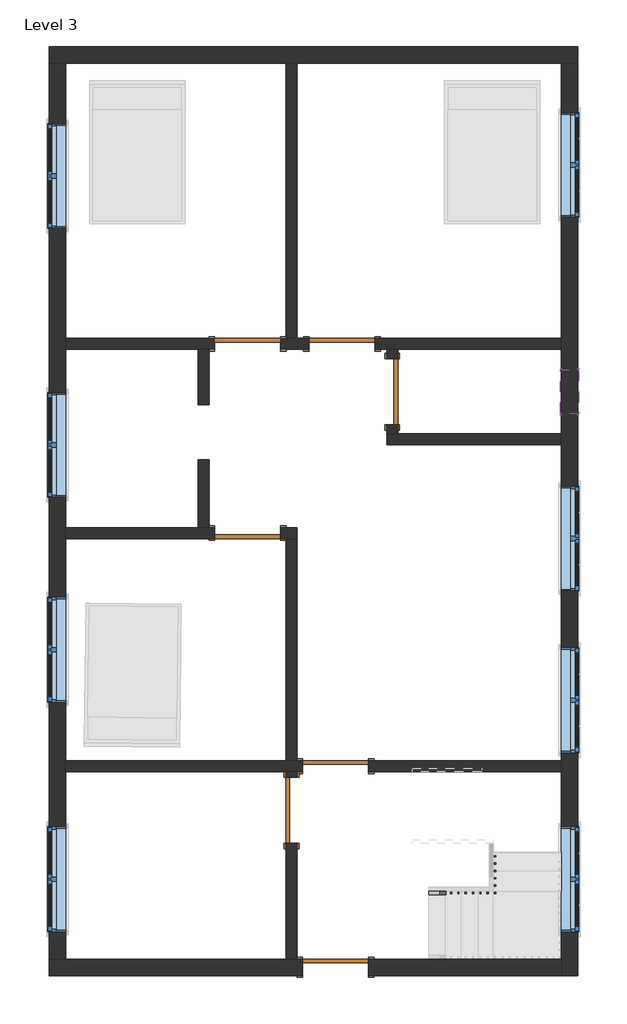
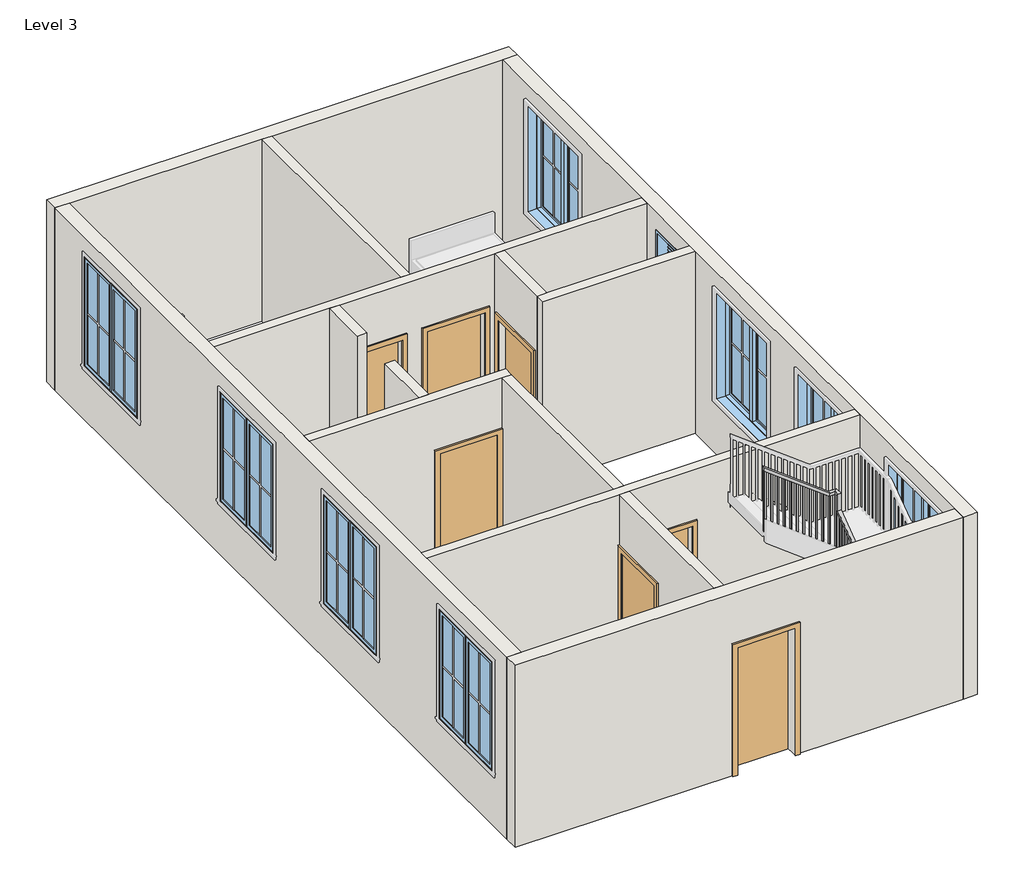
# One storey, part 1 of 2: 14 walls, 9 windows, 7 doors, 1 railing.
"""IFC4 building model written with IfcOpenShell, lengths in millimetres."""

from ifc_helpers import new_model, si_unit, frame, origin, place, context, project, spatial, polyline, outline, extrude, faceted_brep, transform, mapped, element, save
from components import door_2b0b55a0, door_686f89d2, door_16372e1c, door_a90ba1ad, window_9ac97e1a, window_f2d8fef0

model = new_model("IFC4")

# Units and contexts
model_context = context("Model", 3, world=origin())
ifc_project = project(units=[si_unit("LENGTHUNIT", "METRE", prefix="MILLI")], contexts=[model_context])

# Site, building, storey
site = spatial("IfcSite", under=ifc_project)
building = spatial("IfcBuilding", under=site)
storey = spatial("IfcBuildingStorey", under=building, Name="Level 3", Elevation=3200.4)

# Doors
placement = place(None, origin())
door_shape = door_2b0b55a0(model_context)
element("IfcDoor", 1, ObjectType="Single-Flush : 36\" x 80\"", at=placement, inside=storey, context=model_context, shape_type="MappedRepresentation", body=[
    mapped(door_shape, transform((-163.235885, 1707.4649429, 3200.4), x_axis=(0.0, 1.0, 0.0), y_axis=(-1.0, 0.0, 0.0), z_axis=(0.0, 0.0, 1.0))),
])
door_2_shape = door_686f89d2(model_context)
element("IfcDoor", 2, ObjectType="Single-Flush : 36\" x 84\"", at=placement, inside=storey, context=model_context, shape_type="MappedRepresentation", body=[
    mapped(door_2_shape, transform((-861.735885, 2367.8649429, 3200.4), x_axis=(-1.0, 0.0, 0.0), y_axis=(0.0, -1.0, 0.0), z_axis=(0.0, 0.0, 1.0))),
])
element("IfcDoor", 3, ObjectType="Single-Flush : 36\" x 84\"", at=placement, inside=storey, context=model_context, shape_type="MappedRepresentation", body=[
    mapped(door_2_shape, transform((-2169.835885, -248.3350571, 3200.4), x_axis=(1.0, 0.0, 0.0), y_axis=(0.0, 1.0, 0.0), z_axis=(0.0, 0.0, 1.0))),
])
element("IfcDoor", 4, ObjectType="Single-Flush : 36\" x 84\"", at=placement, inside=storey, context=model_context, shape_type="MappedRepresentation", body=[
    mapped(door_2_shape, transform((-950.635885, -3474.1350571, 3200.4), x_axis=(-1.0, 0.0, 0.0), y_axis=(0.0, -1.0, 0.0), z_axis=(0.0, 0.0, 1.0))),
])
door_3_shape = door_16372e1c(model_context)
element("IfcDoor", 5, ObjectType="Single-Flush : 36\" x 84\"", at=placement, inside=storey, context=model_context, shape_type="MappedRepresentation", body=[
    mapped(door_3_shape, transform((-2169.835885, 2367.8649429, 3200.4), x_axis=(1.0, 0.0, 0.0), y_axis=(0.0, 1.0, 0.0), z_axis=(0.0, 0.0, 1.0))),
])
element("IfcDoor", 6, ObjectType="Single-Flush : 36\" x 84\"", at=placement, inside=storey, context=model_context, shape_type="MappedRepresentation", body=[
    mapped(door_3_shape, transform((-1560.235885, -4083.7350571, 3200.4), x_axis=(0.0, 1.0, 0.0), y_axis=(-1.0, 0.0, 0.0), z_axis=(0.0, 0.0, 1.0))),
])
door_4_shape = door_a90ba1ad(model_context)
element("IfcDoor", 7, ObjectType="Single-Flush : 36\" x 84\"", at=placement, inside=storey, context=model_context, shape_type="MappedRepresentation", body=[
    mapped(door_4_shape, transform((-950.635885, -6255.4350571, 3200.4), x_axis=(-1.0, 0.0, 0.0), y_axis=(0.0, -1.0, 0.0), z_axis=(0.0, 0.0, 1.0))),
])

# Railing
element("IfcRailing", 8, ObjectType="Handrail - Rectangular", at=placement, inside=storey, context=model_context, shape_type="SolidModel", body=[
    faceted_brep([(344.764115, -5201.3350571, 4284.1333333), (344.764115, -5201.3350571, 4220.2686436), (344.764115, -5252.1350571, 4220.2686436), (344.764115, -5252.1350571, 4284.1333333), (1157.564115, -5201.3350571, 4903.4095238), (1208.364115, -5201.3350571, 4878.249596), (1208.364115, -5252.1350571, 4878.249596), (1157.564115, -5252.1350571, 4903.4095238), (1157.564115, -5201.3350571, 5185.2285714), (1208.364115, -5201.3350571, 5134.4285714), (1208.364115, -5252.1350571, 5134.4285714), (1157.564115, -5252.1350571, 5185.2285714), (1233.764115, -5201.3350571, 5185.2285714), (1233.764115, -5201.3350571, 5134.4285714), (1284.564115, -5252.1350571, 5134.4285714), (1284.564115, -5252.1350571, 5185.2285714), (1233.764115, -5125.1350571, 5185.2285714), (1233.764115, -5108.8554323, 5134.4285714), (1284.564115, -5108.8554323, 5134.4285714), (1284.564115, -5125.1350571, 5185.2285714), (1233.764115, -4566.3350571, 5584.3714286), (1233.764115, -4515.5350571, 5558.2288395), (1284.564115, -4515.5350571, 5558.2288395), (1284.564115, -4566.3350571, 5584.3714286), (1233.764115, -4566.3350571, 5865.8606061), (1233.764115, -4515.5350571, 5815.0606061), (1284.564115, -4515.5350571, 5815.0606061), (1284.564115, -4566.3350571, 5865.8606061), (1233.764115, -4490.1350571, 5865.8606061), (1233.764115, -4490.1350571, 5815.0606061), (1284.564115, -4439.3350571, 5815.0606061), (1284.564115, -4439.3350571, 5865.8606061), (1157.564115, -4490.1350571, 5865.8606061), (1140.4943334, -4490.1350571, 5815.0606061), (1140.4943334, -4439.3350571, 5815.0606061), (1157.564115, -4439.3350571, 5865.8606061), (116.164115, -4490.1350571, 6654.8), (116.164115, -4439.3350571, 6654.8), (116.164115, -4439.3350571, 6591.0683472), (116.164115, -4490.1350571, 6591.0683472)], [[[0, 1, 2, 3]], [[1, 0, 4, 5]], [[2, 1, 5, 6]], [[3, 2, 6, 7]], [[0, 3, 7, 4]], [[5, 4, 8, 9]], [[6, 5, 9, 10]], [[7, 6, 10, 11]], [[4, 7, 11, 8]], [[9, 8, 12, 13]], [[10, 9, 13, 14]], [[11, 10, 14, 15]], [[8, 11, 15, 12]], [[13, 12, 16, 17]], [[14, 13, 17, 18]], [[15, 14, 18, 19]], [[12, 15, 19, 16]], [[17, 16, 20, 21]], [[18, 17, 21, 22]], [[19, 18, 22, 23]], [[16, 19, 23, 20]], [[21, 20, 24, 25]], [[22, 21, 25, 26]], [[23, 22, 26, 27]], [[20, 23, 27, 24]], [[25, 24, 28, 29]], [[26, 25, 29, 30]], [[27, 26, 30, 31]], [[24, 27, 31, 28]], [[29, 28, 32, 33]], [[30, 29, 33, 34]], [[31, 30, 34, 35]], [[28, 31, 35, 32]], [[36, 37, 38, 39]], [[33, 32, 36, 39]], [[34, 33, 39, 38]], [[35, 34, 38, 37]], [[32, 35, 37, 36]]]),
    extrude(outline(polyline([(6579.0418321, 132.039115), (5571.0666667, 132.039115), (5571.0666667, 151.089115), (6564.6100139, 151.089115), (6579.0418321, 132.039115)])), frame((0.0, -4474.2600571, 0.0), z_axis=(0.0, 1.0, 0.0), x_axis=(0.0, 0.0, 1.0)), (0.0, 0.0, 1.0), 19.05),
    extrude(outline(polyline([(6502.0721351, 233.639115), (5571.0666667, 233.639115), (5571.0666667, 252.689115), (6487.6403169, 252.689115), (6502.0721351, 233.639115)])), frame((0.0, -4474.2600571, 0.0), z_axis=(0.0, 1.0, 0.0), x_axis=(0.0, 0.0, 1.0)), (0.0, 0.0, 1.0), 19.05),
    extrude(outline(polyline([(6425.1024382, 335.239115), (5571.0666667, 335.239115), (5571.0666667, 354.289115), (6410.67062, 354.289115), (6425.1024382, 335.239115)])), frame((0.0, -4474.2600571, 0.0), z_axis=(0.0, 1.0, 0.0), x_axis=(0.0, 0.0, 1.0)), (0.0, 0.0, 1.0), 19.05),
    extrude(outline(polyline([(6348.1327412, 436.839115), (5401.7333333, 436.839115), (5401.7333333, 455.889115), (6333.700923, 455.889115), (6348.1327412, 436.839115)])), frame((0.0, -4474.2600571, 0.0), z_axis=(0.0, 1.0, 0.0), x_axis=(0.0, 0.0, 1.0)), (0.0, 0.0, 1.0), 19.05),
    extrude(outline(polyline([(6271.1630442, 538.439115), (5401.7333333, 538.439115), (5401.7333333, 557.489115), (6256.731226, 557.489115), (6271.1630442, 538.439115)])), frame((0.0, -4474.2600571, 0.0), z_axis=(0.0, 1.0, 0.0), x_axis=(0.0, 0.0, 1.0)), (0.0, 0.0, 1.0), 19.05),
    extrude(outline(polyline([(6194.1933472, 640.039115), (5232.4, 640.039115), (5232.4, 659.089115), (6179.7615291, 659.089115), (6194.1933472, 640.039115)])), frame((0.0, -4474.2600571, 0.0), z_axis=(0.0, 1.0, 0.0), x_axis=(0.0, 0.0, 1.0)), (0.0, 0.0, 1.0), 19.05),
    extrude(outline(polyline([(6117.2236503, 741.639115), (5232.4, 741.639115), (5232.4, 760.689115), (6102.7918321, 760.689115), (6117.2236503, 741.639115)])), frame((0.0, -4474.2600571, 0.0), z_axis=(0.0, 1.0, 0.0), x_axis=(0.0, 0.0, 1.0)), (0.0, 0.0, 1.0), 19.05),
    extrude(outline(polyline([(6040.2539533, 843.239115), (5063.0666667, 843.239115), (5063.0666667, 862.289115), (6025.8221351, 862.289115), (6040.2539533, 843.239115)])), frame((0.0, -4474.2600571, 0.0), z_axis=(0.0, 1.0, 0.0), x_axis=(0.0, 0.0, 1.0)), (0.0, 0.0, 1.0), 19.05),
    extrude(outline(polyline([(5963.2842563, 944.839115), (5063.0666667, 944.839115), (5063.0666667, 963.889115), (5948.8524382, 963.889115), (5963.2842563, 944.839115)])), frame((0.0, -4474.2600571, 0.0), z_axis=(0.0, 1.0, 0.0), x_axis=(0.0, 0.0, 1.0)), (0.0, 0.0, 1.0), 19.05),
    extrude(outline(polyline([(5886.3145594, 1046.439115), (4893.7333333, 1046.439115), (4893.7333333, 1065.489115), (5871.8827412, 1065.489115), (5886.3145594, 1046.439115)])), frame((0.0, -4474.2600571, 0.0), z_axis=(0.0, 1.0, 0.0), x_axis=(0.0, 0.0, 1.0)), (0.0, 0.0, 1.0), 19.05),
    extrude(outline(polyline([(5809.3448624, 1148.039115), (4893.7333333, 1148.039115), (4893.7333333, 1167.089115), (5794.9130442, 1167.089115), (5809.3448624, 1148.039115)])), frame((0.0, -4474.2600571, 0.0), z_axis=(0.0, 1.0, 0.0), x_axis=(0.0, 0.0, 1.0)), (0.0, 0.0, 1.0), 19.05),
    extrude(outline(polyline([(1249.639115, -4525.0600571), (1249.639115, -4506.0100571), (1268.689115, -4506.0100571), (1268.689115, -4525.0600571), (1249.639115, -4525.0600571)])), frame((0.0, 0.0, 4555.0666667), z_axis=(0.0, 0.0, 1.0), x_axis=(1.0, 0.0, 0.0)), (0.0, 0.0, 1.0), 1259.9939394),
    extrude(outline(polyline([(-4607.6100571, 5492.4609823), (-4607.6100571, 4555.0666667), (-4626.6600571, 4555.0666667), (-4626.6600571, 5478.8538395), (-4607.6100571, 5492.4609823)])), frame((1249.639115, 0.0, 0.0), z_axis=(1.0, 0.0, 0.0), x_axis=(0.0, 1.0, 0.0)), (0.0, 0.0, 1.0), 19.05),
    extrude(outline(polyline([(-4709.2100571, 5419.8895538), (-4709.2100571, 4385.7333333), (-4728.2600571, 4385.7333333), (-4728.2600571, 5406.2824109), (-4709.2100571, 5419.8895538)])), frame((1249.639115, 0.0, 0.0), z_axis=(1.0, 0.0, 0.0), x_axis=(0.0, 1.0, 0.0)), (0.0, 0.0, 1.0), 19.05),
    extrude(outline(polyline([(-4810.8100571, 5347.3181252), (-4810.8100571, 4385.7333333), (-4829.8600571, 4385.7333333), (-4829.8600571, 5333.7109823), (-4810.8100571, 5347.3181252)])), frame((1249.639115, 0.0, 0.0), z_axis=(1.0, 0.0, 0.0), x_axis=(0.0, 1.0, 0.0)), (0.0, 0.0, 1.0), 19.05),
    extrude(outline(polyline([(-4912.4100571, 5274.7466966), (-4912.4100571, 4385.7333333), (-4931.4600571, 4385.7333333), (-4931.4600571, 5261.1395538), (-4912.4100571, 5274.7466966)])), frame((1249.639115, 0.0, 0.0), z_axis=(1.0, 0.0, 0.0), x_axis=(0.0, 1.0, 0.0)), (0.0, 0.0, 1.0), 19.05),
    extrude(outline(polyline([(-5014.0100571, 5202.1752681), (-5014.0100571, 4216.4), (-5033.0600571, 4216.4), (-5033.0600571, 5188.5681252), (-5014.0100571, 5202.1752681)])), frame((1249.639115, 0.0, 0.0), z_axis=(1.0, 0.0, 0.0), x_axis=(0.0, 1.0, 0.0)), (0.0, 0.0, 1.0), 19.05),
    extrude(outline(polyline([(-5115.6100571, 5129.6038395), (-5115.6100571, 4216.4), (-5134.6600571, 4216.4), (-5134.6600571, 5115.9966966), (-5115.6100571, 5129.6038395)])), frame((1249.639115, 0.0, 0.0), z_axis=(1.0, 0.0, 0.0), x_axis=(0.0, 1.0, 0.0)), (0.0, 0.0, 1.0), 19.05),
    extrude(outline(polyline([(4832.2876912, 1148.039115), (3877.7333333, 1148.039115), (3877.7333333, 1167.089115), (4846.8019769, 1167.089115), (4832.2876912, 1148.039115)])), frame((0.0, -5236.2600571, 0.0), z_axis=(0.0, 1.0, 0.0), x_axis=(0.0, 0.0, 1.0)), (0.0, 0.0, 1.0), 19.05),
    extrude(outline(polyline([(4754.8781674, 1046.439115), (3877.7333333, 1046.439115), (3877.7333333, 1065.489115), (4769.3924531, 1065.489115), (4754.8781674, 1046.439115)])), frame((0.0, -5236.2600571, 0.0), z_axis=(0.0, 1.0, 0.0), x_axis=(0.0, 0.0, 1.0)), (0.0, 0.0, 1.0), 19.05),
    extrude(outline(polyline([(4677.4686436, 944.839115), (3708.4, 944.839115), (3708.4, 963.889115), (4691.9829293, 963.889115), (4677.4686436, 944.839115)])), frame((0.0, -5236.2600571, 0.0), z_axis=(0.0, 1.0, 0.0), x_axis=(0.0, 0.0, 1.0)), (0.0, 0.0, 1.0), 19.05),
    extrude(outline(polyline([(4600.0591198, 843.239115), (3708.4, 843.239115), (3708.4, 862.289115), (4614.5734055, 862.289115), (4600.0591198, 843.239115)])), frame((0.0, -5236.2600571, 0.0), z_axis=(0.0, 1.0, 0.0), x_axis=(0.0, 0.0, 1.0)), (0.0, 0.0, 1.0), 19.05),
    extrude(outline(polyline([(4522.649596, 741.639115), (3539.0666667, 741.639115), (3539.0666667, 760.689115), (4537.1638817, 760.689115), (4522.649596, 741.639115)])), frame((0.0, -5236.2600571, 0.0), z_axis=(0.0, 1.0, 0.0), x_axis=(0.0, 0.0, 1.0)), (0.0, 0.0, 1.0), 19.05),
    extrude(outline(polyline([(4445.2400722, 640.039115), (3539.0666667, 640.039115), (3539.0666667, 659.089115), (4459.7543579, 659.089115), (4445.2400722, 640.039115)])), frame((0.0, -5236.2600571, 0.0), z_axis=(0.0, 1.0, 0.0), x_axis=(0.0, 0.0, 1.0)), (0.0, 0.0, 1.0), 19.05),
    extrude(outline(polyline([(4367.8305484, 538.439115), (3369.7333333, 538.439115), (3369.7333333, 557.489115), (4382.3448341, 557.489115), (4367.8305484, 538.439115)])), frame((0.0, -5236.2600571, 0.0), z_axis=(0.0, 1.0, 0.0), x_axis=(0.0, 0.0, 1.0)), (0.0, 0.0, 1.0), 19.05),
    extrude(outline(polyline([(4290.4210246, 436.839115), (3369.7333333, 436.839115), (3369.7333333, 455.889115), (4304.9353103, 455.889115), (4290.4210246, 436.839115)])), frame((0.0, -5236.2600571, 0.0), z_axis=(0.0, 1.0, 0.0), x_axis=(0.0, 0.0, 1.0)), (0.0, 0.0, 1.0), 19.05),
    extrude(outline(polyline([(1249.639115, -4474.2600571), (1249.639115, -4455.2100571), (1268.689115, -4455.2100571), (1268.689115, -4474.2600571), (1249.639115, -4474.2600571)])), frame((0.0, 0.0, 4724.4), z_axis=(0.0, 0.0, 1.0), x_axis=(1.0, 0.0, 0.0)), (0.0, 0.0, 1.0), 1090.6606061),
    extrude(outline(polyline([(1249.639115, -5217.2100571), (1268.689115, -5217.2100571), (1268.689115, -5236.2600571), (1249.639115, -5236.2600571), (1249.639115, -5217.2100571)])), frame((0.0, 0.0, 4047.0666667), z_axis=(0.0, 0.0, 1.0), x_axis=(1.0, 0.0, 0.0)), (0.0, 0.0, 1.0), 1087.3619048),
    extrude(outline(polyline([(6591.0683472, 116.164115), (5571.0666667, 116.164115), (5571.0666667, 135.214115), (6576.6365291, 135.214115), (6591.0683472, 116.164115)])), frame((0.0, -4474.2600571, 0.0), z_axis=(0.0, 1.0, 0.0), x_axis=(0.0, 0.0, 1.0)), (0.0, 0.0, 1.0), 19.05),
    extrude(outline(polyline([(4220.2686436, 344.764115), (3369.7333333, 344.764115), (3369.7333333, 363.814115), (4234.7829293, 363.814115), (4220.2686436, 344.764115)])), frame((0.0, -5236.2600571, 0.0), z_axis=(0.0, 1.0, 0.0), x_axis=(0.0, 0.0, 1.0)), (0.0, 0.0, 1.0), 19.05),
])

# Walls
element("IfcWall", 9, ObjectType="WALL 6\"", at=placement, inside=storey, context=model_context, shape_type="SweptSolid", body=[
    extrude(outline(polyline([(-1636.435885, 2444.0649429), (-1636.435885, 6254.0649429), (-1484.035885, 6254.0649429), (-1484.035885, 2444.0649429), (-1636.435885, 2444.0649429)])), frame((0.0, 0.0, 3200.4), z_axis=(0.0, 0.0, 1.0), x_axis=(1.0, 0.0, 0.0)), (0.0, 0.0, 1.0), 3048.0),
])
element("IfcWall", 10, ObjectType="WALL 6\"", at=placement, inside=storey, context=model_context, shape_type="Brep", body=[
    faceted_brep([(-1318.935885, 2444.0649429, 3200.4), (-1484.035885, 2444.0649429, 3200.4), (-1636.435885, 2444.0649429, 3200.4), (-1712.635885, 2444.0649429, 3200.4), (-1712.635885, 2444.0649429, 5334.0), (-2627.035885, 2444.0649429, 5334.0), (-2627.035885, 2444.0649429, 3200.4), (-4684.435885, 2444.0649429, 3200.4), (-4684.435885, 2444.0649429, 6248.4), (-1636.435885, 2444.0649429, 6248.4), (-1484.035885, 2444.0649429, 6248.4), (2173.564115, 2444.0649429, 6248.4), (2173.564115, 2444.0649429, 3200.4), (-404.535885, 2444.0649429, 3200.4), (-404.535885, 2444.0649429, 5334.0), (-1318.935885, 2444.0649429, 5334.0), (-1712.635885, 2291.6649429, 5334.0), (-1712.635885, 2291.6649429, 3200.4), (-1318.935885, 2291.6649429, 3200.4), (-1318.935885, 2291.6649429, 5334.0), (-404.535885, 2291.6649429, 5334.0), (-404.535885, 2291.6649429, 3200.4), (-239.435885, 2291.6649429, 3200.4), (-87.035885, 2291.6649429, 3200.4), (2173.564115, 2291.6649429, 3200.4), (2173.564115, 2291.6649429, 6248.4), (-87.035885, 2291.6649429, 6248.4), (-239.435885, 2291.6649429, 6248.4), (-2703.235885, 2291.6649429, 6248.4), (-2855.635885, 2291.6649429, 6248.4), (-4684.435885, 2291.6649429, 6248.4), (-4684.435885, 2291.6649429, 3200.4), (-2855.635885, 2291.6649429, 3200.4), (-2703.235885, 2291.6649429, 3200.4), (-2627.035885, 2291.6649429, 3200.4), (-2627.035885, 2291.6649429, 5334.0)], [[[0, 1, 2, 3, 4, 5, 6, 7, 8, 9, 10, 11, 12, 13, 14, 15]], [[16, 17, 18, 19, 20, 21, 22, 23, 24, 25, 26, 27, 28, 29, 30, 31, 32, 33, 34, 35]], [[13, 12, 24, 23, 22, 21]], [[18, 17, 3, 2, 1, 0]], [[34, 33, 32, 31, 7, 6]], [[12, 11, 25, 24]], [[8, 7, 31, 30]], [[19, 18, 0, 15]], [[20, 19, 15, 14]], [[21, 20, 14, 13]], [[4, 3, 17, 16]], [[5, 4, 16, 35]], [[6, 5, 35, 34]], [[11, 10, 9, 8, 30, 29, 28, 27, 26, 25]]]),
])
element("IfcWall", 11, ObjectType="WALL 6\"", at=placement, inside=storey, context=model_context, shape_type="SweptSolid", body=[
    extrude(outline(polyline([(-2855.635885, 1529.6649429), (-2855.635885, 2291.6649429), (-2703.235885, 2291.6649429), (-2703.235885, 1529.6649429), (-2855.635885, 1529.6649429)])), frame((0.0, 0.0, 3200.4), z_axis=(0.0, 0.0, 1.0), x_axis=(1.0, 0.0, 0.0)), (0.0, 0.0, 1.0), 3048.0),
])
element("IfcWall", 12, ObjectType="WALL 6\"", at=placement, inside=storey, context=model_context, shape_type="Brep", body=[
    faceted_brep([(-1712.635885, -324.5350571, 5334.0), (-1712.635885, -324.5350571, 3200.4), (-1636.435885, -324.5350571, 3200.4), (-1484.035885, -324.5350571, 3200.4), (-1484.035885, -324.5350571, 6248.4), (-1636.435885, -324.5350571, 6248.4), (-4684.435885, -324.5350571, 6248.4), (-4684.435885, -324.5350571, 3200.4), (-2627.035885, -324.5350571, 3200.4), (-2627.035885, -324.5350571, 5334.0), (-1484.035885, -172.1350571, 3200.4), (-1712.635885, -172.1350571, 3200.4), (-1712.635885, -172.1350571, 5334.0), (-2627.035885, -172.1350571, 5334.0), (-2627.035885, -172.1350571, 3200.4), (-2703.235885, -172.1350571, 3200.4), (-2855.635885, -172.1350571, 3200.4), (-4684.435885, -172.1350571, 3200.4), (-4684.435885, -172.1350571, 6248.4), (-2855.635885, -172.1350571, 6248.4), (-2703.235885, -172.1350571, 6248.4), (-1484.035885, -172.1350571, 6248.4)], [[[0, 1, 2, 3, 4, 5, 6, 7, 8, 9]], [[10, 11, 12, 13, 14, 15, 16, 17, 18, 19, 20, 21]], [[8, 7, 17, 16, 15, 14]], [[3, 2, 1, 11, 10]], [[7, 6, 18, 17]], [[4, 3, 10, 21]], [[12, 11, 1, 0]], [[13, 12, 0, 9]], [[14, 13, 9, 8]], [[6, 5, 4, 21, 20, 19, 18]]]),
])
element("IfcWall", 13, ObjectType="WALL 6\"", at=placement, inside=storey, context=model_context, shape_type="SweptSolid", body=[
    extrude(outline(polyline([(-1636.435885, -3397.9350571), (-1636.435885, -324.5350571), (-1484.035885, -324.5350571), (-1484.035885, -3397.9350571), (-1636.435885, -3397.9350571)])), frame((0.0, 0.0, 3200.4), z_axis=(0.0, 0.0, 1.0), x_axis=(1.0, 0.0, 0.0)), (0.0, 0.0, 1.0), 3048.0),
])
element("IfcWall", 14, ObjectType="WALL 6\"", at=placement, inside=storey, context=model_context, shape_type="Brep", body=[
    faceted_brep([(-4684.435885, -3550.3350571, 3200.4), (-1636.435885, -3550.3350571, 3200.4), (-1484.035885, -3550.3350571, 3200.4), (-1407.835885, -3550.3350571, 3200.4), (-1407.835885, -3550.3350571, 5334.0), (-493.435885, -3550.3350571, 5334.0), (-493.435885, -3550.3350571, 3200.4), (2173.564115, -3550.3350571, 3200.4), (2173.564115, -3550.3350571, 6248.4), (-1484.035885, -3550.3350571, 6248.4), (-1636.435885, -3550.3350571, 6248.4), (-4684.435885, -3550.3350571, 6248.4), (-1407.835885, -3397.9350571, 5334.0), (-1407.835885, -3397.9350571, 3200.4), (-1484.035885, -3397.9350571, 3200.4), (-1636.435885, -3397.9350571, 3200.4), (-4684.435885, -3397.9350571, 3200.4), (-4684.435885, -3397.9350571, 6248.4), (-1636.435885, -3397.9350571, 6248.4), (-1484.035885, -3397.9350571, 6248.4), (2173.564115, -3397.9350571, 6248.4), (2173.564115, -3397.9350571, 3200.4), (-493.435885, -3397.9350571, 3200.4), (-493.435885, -3397.9350571, 5334.0)], [[[0, 1, 2, 3, 4, 5, 6, 7, 8, 9, 10, 11]], [[12, 13, 14, 15, 16, 17, 18, 19, 20, 21, 22, 23]], [[22, 21, 7, 6]], [[16, 15, 14, 13, 3, 2, 1, 0]], [[8, 7, 21, 20]], [[0, 11, 17, 16]], [[4, 3, 13, 12]], [[5, 4, 12, 23]], [[6, 5, 23, 22]], [[11, 10, 9, 8, 20, 19, 18, 17]]]),
])
element("IfcWall", 15, ObjectType="WALL 6\"", at=placement, inside=storey, context=model_context, shape_type="SweptSolid", body=[
    extrude(outline(polyline([(-3550.3350571, 3200.4), (-3626.5350571, 3200.4), (-3626.5350571, 5334.0), (-4540.9350571, 5334.0), (-4540.9350571, 3200.4), (-6141.1350571, 3200.4), (-6141.1350571, 6248.4), (-3550.3350571, 6248.4), (-3550.3350571, 3200.4)])), frame((-1636.435885, 0.0, 0.0), z_axis=(1.0, 0.0, 0.0), x_axis=(0.0, 1.0, 0.0)), (0.0, 0.0, 1.0), 152.4),
])
element("IfcWall", 16, ObjectType="WALL 6\"", at=placement, inside=storey, context=model_context, shape_type="Brep", body=[
    faceted_brep([(2173.564115, 1123.2649429, 3200.4), (-87.035885, 1123.2649429, 3200.4), (-239.435885, 1123.2649429, 3200.4), (-239.435885, 1123.2649429, 6248.4), (-87.035885, 1123.2649429, 6248.4), (2173.564115, 1123.2649429, 6248.4), (2173.564115, 970.8649429, 3200.4), (2173.564115, 970.8649429, 6248.4), (-239.435885, 970.8649429, 6248.4), (-239.435885, 970.8649429, 3200.4)], [[[0, 1, 2, 3, 4, 5]], [[6, 7, 8, 9]], [[2, 1, 0, 6, 9]], [[0, 5, 7, 6]], [[3, 2, 9, 8]], [[5, 4, 3, 8, 7]]]),
])
element("IfcWall", 17, ObjectType="WALL 6\"", at=placement, inside=storey, context=model_context, shape_type="SweptSolid", body=[
    extrude(outline(polyline([(2291.6649429, 3200.4), (2164.6649429, 3200.4), (2164.6649429, 5232.4), (1250.2649429, 5232.4), (1250.2649429, 3200.4), (1123.2649429, 3200.4), (1123.2649429, 6248.4), (2291.6649429, 6248.4), (2291.6649429, 3200.4)])), frame((-239.435885, 0.0, 0.0), z_axis=(1.0, 0.0, 0.0), x_axis=(0.0, 1.0, 0.0)), (0.0, 0.0, 1.0), 152.4),
])
element("IfcWall", 18, ObjectType="WALL 6\"", at=placement, inside=storey, context=model_context, shape_type="SweptSolid", body=[
    extrude(outline(polyline([(-2855.635885, -172.1350571), (-2855.635885, 767.6649429), (-2703.235885, 767.6649429), (-2703.235885, -172.1350571), (-2855.635885, -172.1350571)])), frame((0.0, 0.0, 3200.4), z_axis=(0.0, 0.0, 1.0), x_axis=(1.0, 0.0, 0.0)), (0.0, 0.0, 1.0), 3048.0),
])
element("IfcWall", 19, ObjectType="WALL 9\"", at=placement, inside=storey, context=model_context, shape_type="Brep", body=[
    faceted_brep([(-4913.035885, 6254.0649429, 3200.4), (-4684.435885, 6254.0649429, 3200.4), (-1636.435885, 6254.0649429, 3200.4), (-1484.035885, 6254.0649429, 3200.4), (2173.564115, 6254.0649429, 3200.4), (2402.164115, 6254.0649429, 3200.4), (2402.164115, 6254.0649429, 6248.4), (2173.564115, 6254.0649429, 6248.4), (-1484.035885, 6254.0649429, 6248.4), (-1636.435885, 6254.0649429, 6248.4), (-4684.435885, 6254.0649429, 6248.4), (-4913.035885, 6254.0649429, 6248.4), (-4913.035885, 6482.6649429, 3200.4), (-4913.035885, 6482.6649429, 6248.4), (2402.164115, 6482.6649429, 6248.4), (2402.164115, 6482.6649429, 3200.4)], [[[0, 1, 2, 3, 4, 5, 6, 7, 8, 9, 10, 11]], [[12, 13, 14, 15]], [[5, 4, 3, 2, 1, 0, 12, 15]], [[6, 5, 15, 14]], [[0, 11, 13, 12]], [[11, 10, 9, 8, 7, 6, 14, 13]]]),
])
element("IfcWall", 20, ObjectType="WALL 9\"", at=placement, inside=storey, context=model_context, shape_type="Brep", body=[
    faceted_brep([(2173.564115, 6254.0649429, 3200.4), (2173.564115, 2444.0649429, 3200.4), (2173.564115, 2291.6649429, 3200.4), (2173.564115, 1123.2649429, 3200.4), (2173.564115, 970.8649429, 3200.4), (2173.564115, -3397.9350571, 3200.4), (2173.564115, -3550.3350571, 3200.4), (2173.564115, -6141.1350571, 3200.4), (2173.564115, -6369.7350571, 3200.4), (2173.564115, -6369.7350571, 6248.4), (2173.564115, -6141.1350571, 6248.4), (2173.564115, -3550.3350571, 6248.4), (2173.564115, -3397.9350571, 6248.4), (2173.564115, 970.8649429, 6248.4), (2173.564115, 1123.2649429, 6248.4), (2173.564115, 2291.6649429, 6248.4), (2173.564115, 2444.0649429, 6248.4), (2173.564115, 6254.0649429, 6248.4), (2173.564115, -5760.1350571, 5943.6), (2173.564115, -5760.1350571, 4114.8), (2173.564115, -4312.3350571, 4114.8), (2173.564115, -4312.3350571, 5943.6), (2173.564115, -3283.6350571, 5943.6), (2173.564115, -3283.6350571, 4114.8), (2173.564115, -1835.8350571, 4114.8), (2173.564115, -1835.8350571, 5943.6), (2173.564115, -1048.4350571, 5943.6), (2173.564115, -1048.4350571, 4114.8), (2173.564115, 399.3649429, 4114.8), (2173.564115, 399.3649429, 5943.6), (2173.564115, 4120.4649429, 5943.6), (2173.564115, 4120.4649429, 4114.8), (2173.564115, 5568.2649429, 4114.8), (2173.564115, 5568.2649429, 5943.6), (2173.564115, 2012.2649429, 5943.6), (2173.564115, 1402.6649429, 5943.6), (2173.564115, 1402.6649429, 5334.0), (2173.564115, 2012.2649429, 5334.0), (2402.164115, 6254.0649429, 3200.4), (2402.164115, 6254.0649429, 6248.4), (2402.164115, -6369.7350571, 6248.4), (2402.164115, -6369.7350571, 3200.4), (2402.164115, -5760.1350571, 5943.6), (2402.164115, -4312.3350571, 5943.6), (2402.164115, -4312.3350571, 4114.8), (2402.164115, -5760.1350571, 4114.8), (2402.164115, -3283.6350571, 5943.6), (2402.164115, -1835.8350571, 5943.6), (2402.164115, -1835.8350571, 4114.8), (2402.164115, -3283.6350571, 4114.8), (2402.164115, -1048.4350571, 5943.6), (2402.164115, 399.3649429, 5943.6), (2402.164115, 399.3649429, 4114.8), (2402.164115, -1048.4350571, 4114.8), (2402.164115, 4120.4649429, 5943.6), (2402.164115, 5568.2649429, 5943.6), (2402.164115, 5568.2649429, 4114.8), (2402.164115, 4120.4649429, 4114.8), (2402.164115, 2012.2649429, 5943.6), (2402.164115, 2012.2649429, 5334.0), (2402.164115, 1402.6649429, 5334.0), (2402.164115, 1402.6649429, 5943.6)], [[[0, 1, 2, 3, 4, 5, 6, 7, 8, 9, 10, 11, 12, 13, 14, 15, 16, 17], [18, 19, 20, 21], [22, 23, 24, 25], [26, 27, 28, 29], [30, 31, 32, 33], [34, 35, 36, 37]], [[38, 39, 40, 41], [42, 43, 44, 45], [46, 47, 48, 49], [50, 51, 52, 53], [54, 55, 56, 57], [58, 59, 60, 61]], [[8, 7, 6, 5, 4, 3, 2, 1, 0, 38, 41]], [[0, 17, 39, 38]], [[9, 8, 41, 40]], [[19, 18, 42, 45]], [[20, 19, 45, 44]], [[21, 20, 44, 43]], [[18, 21, 43, 42]], [[23, 22, 46, 49]], [[24, 23, 49, 48]], [[25, 24, 48, 47]], [[22, 25, 47, 46]], [[27, 26, 50, 53]], [[28, 27, 53, 52]], [[29, 28, 52, 51]], [[26, 29, 51, 50]], [[31, 30, 54, 57]], [[32, 31, 57, 56]], [[33, 32, 56, 55]], [[30, 33, 55, 54]], [[59, 58, 34, 37]], [[60, 59, 37, 36]], [[61, 60, 36, 35]], [[58, 61, 35, 34]], [[17, 16, 15, 14, 13, 12, 11, 10, 9, 40, 39]]]),
])
element("IfcWall", 21, ObjectType="WALL 9\"", at=placement, inside=storey, context=model_context, shape_type="Brep", body=[
    faceted_brep([(-1407.835885, -6141.1350571, 5334.0), (-1407.835885, -6141.1350571, 3200.4), (-1484.035885, -6141.1350571, 3200.4), (-1636.435885, -6141.1350571, 3200.4), (-4684.435885, -6141.1350571, 3200.4), (-4913.035885, -6141.1350571, 3200.4), (-4913.035885, -6141.1350571, 6248.4), (-4684.435885, -6141.1350571, 6248.4), (-1636.435885, -6141.1350571, 6248.4), (-1484.035885, -6141.1350571, 6248.4), (2173.564115, -6141.1350571, 6248.4), (2173.564115, -6141.1350571, 3200.4), (-493.435885, -6141.1350571, 3200.4), (-493.435885, -6141.1350571, 5334.0), (-4913.035885, -6369.7350571, 3200.4), (-1407.835885, -6369.7350571, 3200.4), (-1407.835885, -6369.7350571, 5334.0), (-493.435885, -6369.7350571, 5334.0), (-493.435885, -6369.7350571, 3200.4), (2173.564115, -6369.7350571, 3200.4), (2173.564115, -6369.7350571, 6248.4), (-4913.035885, -6369.7350571, 6248.4)], [[[0, 1, 2, 3, 4, 5, 6, 7, 8, 9, 10, 11, 12, 13]], [[14, 15, 16, 17, 18, 19, 20, 21]], [[12, 11, 19, 18]], [[5, 4, 3, 2, 1, 15, 14]], [[11, 10, 20, 19]], [[6, 5, 14, 21]], [[16, 15, 1, 0]], [[17, 16, 0, 13]], [[18, 17, 13, 12]], [[10, 9, 8, 7, 6, 21, 20]]]),
])
element("IfcWall", 22, ObjectType="WALL 9\"", at=placement, inside=storey, context=model_context, shape_type="Brep", body=[
    faceted_brep([(-4684.435885, -6141.1350571, 3200.4), (-4684.435885, -3550.3350571, 3200.4), (-4684.435885, -3397.9350571, 3200.4), (-4684.435885, -324.5350571, 3200.4), (-4684.435885, -172.1350571, 3200.4), (-4684.435885, 2291.6649429, 3200.4), (-4684.435885, 2444.0649429, 3200.4), (-4684.435885, 6254.0649429, 3200.4), (-4684.435885, 6254.0649429, 6248.4), (-4684.435885, 2444.0649429, 6248.4), (-4684.435885, 2291.6649429, 6248.4), (-4684.435885, -172.1350571, 6248.4), (-4684.435885, -324.5350571, 6248.4), (-4684.435885, -3397.9350571, 6248.4), (-4684.435885, -3550.3350571, 6248.4), (-4684.435885, -6141.1350571, 6248.4), (-4684.435885, -4312.3350571, 5943.6), (-4684.435885, -4312.3350571, 4114.8), (-4684.435885, -5760.1350571, 4114.8), (-4684.435885, -5760.1350571, 5943.6), (-4684.435885, -1137.3350571, 5943.6), (-4684.435885, -1137.3350571, 4114.8), (-4684.435885, -2585.1350571, 4114.8), (-4684.435885, -2585.1350571, 5943.6), (-4684.435885, 1694.7649429, 5943.6), (-4684.435885, 1694.7649429, 4114.8), (-4684.435885, 246.9649429, 4114.8), (-4684.435885, 246.9649429, 5943.6), (-4684.435885, 5415.8649429, 5943.6), (-4684.435885, 5415.8649429, 4114.8), (-4684.435885, 3968.0649429, 4114.8), (-4684.435885, 3968.0649429, 5943.6), (-4913.035885, -6141.1350571, 3200.4), (-4913.035885, -6141.1350571, 6248.4), (-4913.035885, 6254.0649429, 6248.4), (-4913.035885, 6254.0649429, 3200.4), (-4913.035885, -4312.3350571, 5943.6), (-4913.035885, -5760.1350571, 5943.6), (-4913.035885, -5760.1350571, 4114.8), (-4913.035885, -4312.3350571, 4114.8), (-4913.035885, -1137.3350571, 5943.6), (-4913.035885, -2585.1350571, 5943.6), (-4913.035885, -2585.1350571, 4114.8), (-4913.035885, -1137.3350571, 4114.8), (-4913.035885, 1694.7649429, 5943.6), (-4913.035885, 246.9649429, 5943.6), (-4913.035885, 246.9649429, 4114.8), (-4913.035885, 1694.7649429, 4114.8), (-4913.035885, 5415.8649429, 5943.6), (-4913.035885, 3968.0649429, 5943.6), (-4913.035885, 3968.0649429, 4114.8), (-4913.035885, 5415.8649429, 4114.8)], [[[0, 1, 2, 3, 4, 5, 6, 7, 8, 9, 10, 11, 12, 13, 14, 15], [16, 17, 18, 19], [20, 21, 22, 23], [24, 25, 26, 27], [28, 29, 30, 31]], [[32, 33, 34, 35], [36, 37, 38, 39], [40, 41, 42, 43], [44, 45, 46, 47], [48, 49, 50, 51]], [[7, 6, 5, 4, 3, 2, 1, 0, 32, 35]], [[8, 7, 35, 34]], [[0, 15, 33, 32]], [[17, 16, 36, 39]], [[18, 17, 39, 38]], [[19, 18, 38, 37]], [[16, 19, 37, 36]], [[21, 20, 40, 43]], [[22, 21, 43, 42]], [[23, 22, 42, 41]], [[20, 23, 41, 40]], [[25, 24, 44, 47]], [[26, 25, 47, 46]], [[27, 26, 46, 45]], [[24, 27, 45, 44]], [[29, 28, 48, 51]], [[30, 29, 51, 50]], [[31, 30, 50, 49]], [[28, 31, 49, 48]], [[15, 14, 13, 12, 11, 10, 9, 8, 34, 33]]]),
])

# Windows
window_shape = window_9ac97e1a(model_context)
element("IfcWindow", 23, ObjectType="Window-Casement-Double : 57\" x 72\"", at=placement, inside=storey, context=model_context, shape_type="MappedRepresentation", body=[
    mapped(window_shape, transform((-4798.735885, -5036.2350571, 3200.4), x_axis=(0.0, 1.0, 0.0), y_axis=(-1.0, 0.0, 0.0), z_axis=(0.0, 0.0, 1.0))),
])
element("IfcWindow", 24, ObjectType="Window-Casement-Double : 57\" x 72\"", at=placement, inside=storey, context=model_context, shape_type="MappedRepresentation", body=[
    mapped(window_shape, transform((2287.864115, -5036.2350571, 3200.4), x_axis=(0.0, -1.0, 0.0), y_axis=(1.0, 0.0, 0.0), z_axis=(0.0, 0.0, 1.0))),
])
element("IfcWindow", 25, ObjectType="Window-Casement-Double : 57\" x 72\"", at=placement, inside=storey, context=model_context, shape_type="MappedRepresentation", body=[
    mapped(window_shape, transform((2287.864115, -2559.7350571, 3200.4), x_axis=(0.0, -1.0, 0.0), y_axis=(1.0, 0.0, 0.0), z_axis=(0.0, 0.0, 1.0))),
])
element("IfcWindow", 26, ObjectType="Window-Casement-Double : 57\" x 72\"", at=placement, inside=storey, context=model_context, shape_type="MappedRepresentation", body=[
    mapped(window_shape, transform((2287.864115, -324.5350571, 3200.4), x_axis=(0.0, -1.0, 0.0), y_axis=(1.0, 0.0, 0.0), z_axis=(0.0, 0.0, 1.0))),
])
element("IfcWindow", 27, ObjectType="Window-Casement-Double : 57\" x 72\"", at=placement, inside=storey, context=model_context, shape_type="MappedRepresentation", body=[
    mapped(window_shape, transform((-4798.735885, -1861.2350571, 3200.4), x_axis=(0.0, 1.0, 0.0), y_axis=(-1.0, 0.0, 0.0), z_axis=(0.0, 0.0, 1.0))),
])
element("IfcWindow", 28, ObjectType="Window-Casement-Double : 57\" x 72\"", at=placement, inside=storey, context=model_context, shape_type="MappedRepresentation", body=[
    mapped(window_shape, transform((-4798.735885, 970.8649429, 3200.4), x_axis=(0.0, 1.0, 0.0), y_axis=(-1.0, 0.0, 0.0), z_axis=(0.0, 0.0, 1.0))),
])
element("IfcWindow", 29, ObjectType="Window-Casement-Double : 57\" x 72\"", at=placement, inside=storey, context=model_context, shape_type="MappedRepresentation", body=[
    mapped(window_shape, transform((-4798.735885, 4691.9649429, 3200.4), x_axis=(0.0, 1.0, 0.0), y_axis=(-1.0, 0.0, 0.0), z_axis=(0.0, 0.0, 1.0))),
])
element("IfcWindow", 30, ObjectType="Window-Casement-Double : 57\" x 72\"", at=placement, inside=storey, context=model_context, shape_type="MappedRepresentation", body=[
    mapped(window_shape, transform((2287.864115, 4844.3649429, 3200.4), x_axis=(0.0, -1.0, 0.0), y_axis=(1.0, 0.0, 0.0), z_axis=(0.0, 0.0, 1.0))),
])
window_2_shape = window_f2d8fef0(model_context)
element("IfcWindow", 31, ObjectType="Window-Louvers : 24\" x 24\"", at=placement, inside=storey, context=model_context, shape_type="MappedRepresentation", body=[
    mapped(window_2_shape, transform((2294.214115, 1707.4649429, 4419.6), x_axis=(0.0, -1.0, 0.0), y_axis=(1.0, 0.0, 0.0), z_axis=(0.0, 0.0, 1.0))),
])

save(model, "model.ifc")

# Revit data of these elements
# Type "Single-Flush : 36\" x 80\""
#   Type Mark = "6"
#   Construction Type Id = "MDOOR"
#   Assembly Code = "C1020"
#   Analytic Construction = "Metal"
#   Thickness = 0' - 2"
#   Heat Transfer Coefficient (U) = 0.651978 BTU/(h·ft²·°F)
#   Height = 6' - 8"
#   Trim Projection Ext = 0' - 1"
#   Trim Projection Int = 0' - 1"
#   Trim Width = 0' - 3"
#   Width = 3' - 0"
#   Define Thermal Properties by = 1
#   Define Thermal Properties by = 1
#   Door Material = Door - Panel
#   Frame Material = Door - Frame
#   Visual Light Transmittance = 0
#   Solar Heat Gain Coefficient = 0
#   Function = (empty or 0)
#   Wall Closure = (empty or 0)
# Type "Single-Flush : 36\" x 84\""
#   Type Mark = "1"
#   Construction Type Id = "MDOOR"
#   Assembly Code = "C1020"
#   Analytic Construction = "Metal"
#   Thickness = 0' - 2"
#   Heat Transfer Coefficient (U) = 0.651978 BTU/(h·ft²·°F)
#   Height = 7' - 0"
#   Trim Projection Ext = 0' - 1"
#   Trim Projection Int = 0' - 1"
#   Trim Width = 0' - 3"
#   Width = 3' - 0"
#   Define Thermal Properties by = 1
#   Define Thermal Properties by = 1
#   Door Material = Door - Panel
#   Frame Material = Door - Frame
#   Visual Light Transmittance = 0
#   Solar Heat Gain Coefficient = 0
#   Function = (empty or 0)
#   Wall Closure = (empty or 0)
# Type "Handrail - Rectangular"
#   Assembly Code = "C2010400"
#   built-in parameter 1008612 = 0.0416667 (stored number, unit not read)
#   built-in parameter 1008611 = 0.0416667 (stored number, unit not read)
#   built-in parameter 1008609 = 0.333333 (stored number, unit not read)
#   built-in parameter 1008604 = 0.166667 (stored number, unit not read)
#   built-in parameter 1008603 = 0.166667 (stored number, unit not read)
#   Railing Height = 3' - 0"
#   built-in parameter 1008630 = 2
#   built-in parameter 1008610 = 2
#   built-in parameter 1008618 = Baluster - Square : 3/4"
# Type "WALL 6\""
#   Assembly Code = "B2010"
#   Layers, outside or top first: 0' - 6" no material (function 1)
# Type "WALL 9\""
#   Assembly Code = "B2010"
#   Layers, outside or top first: 0' - 9" no material (function 1)
# Type "Window-Casement-Double : 57\" x 72\""
#   Type Mark = "17"
#   Fire Rating = "0.5h"
#   Assembly Code = "B2020100"
#   Analytic Construction = "Double glazing - domestic"
#   Frame Extension [instance default] = 0' - 0 1/4"
#   Window Inset [instance default] = 0' - 0"
#   Wall Thickness [instance default] = 0' - 6"
#   Interior Wall Closure [instance default] = 0' - 2 1/4"
#   Half Width = 2' - 4 1/2"
#   Visual Light Transmittance = 0.81
#   Thermal Resistance (R) = 1.8146 (h·ft²·°F)/BTU
#   Solar Heat Gain Coefficient = 0.76
#   Rough Width = 4' - 9 1/2"
#   Rough Height = 6' - 0 1/2"
#   Height = 6' - 0"
#   Heat Transfer Coefficient (U) = 0.5511 BTU/(h·ft²·°F)
#   Exterior Wall Closure [instance default] = 0' - 1 1/4"
#   Extension Jamb [instance default] = 0' - 2 1/4"
#   Default Sill Height = 3' - 0"
#   Width = 4' - 9"
#   Define Thermal Properties by = 0
#   Muntin Visibility = yes
#   Interior Trim Visibility [instance default] = yes
#   Exterior Trim Visibility [instance default] = yes
#   Extension Jamb Visibility [instance default] = yes
#   Interior Trim Material = Wood - Stained
#   Muntin Pattern = Muntin Pattern_2x2 : Muntin Pattern_2x2
#   Interior Trim = Trim-Window-Interior-Flat : Picture Frame
#   Interior Frame Material = Wood - Stained
#   Glass Panel Material = Glass
#   Exterior Trim Material = Clad - White
#   Exterior Trim = Trim-Window-Exterior-Flat : with Sill
#   Exterior Frame Material = Clad - White
#   Wall Closure = (empty or 0)
# Type "Window-Louvers : 24\" x 24\""
#   Type Mark = "18"
#   Construction Type Id = "GSP4R"
#   Assembly Code = "B20"
#   Analytic Construction = "1/8 in Pilkington single glazing"
#   Visual Light Transmittance = 0.9
#   Thermal Resistance (R) = 1.53941 (h·ft²·°F)/BTU
#   Solar Heat Gain Coefficient = 0.78
#   Max Height = 1' - 11.74264"
#   Height = 2' - 0"
#   Heat Transfer Coefficient (U) = 0.6496 BTU/(h·ft²·°F)
#   Blade Width [instance default] = 1' - 10 1/2"
#   Blade Vertical Thickness = 0' - 0.35355"
#   Blade Thickness = 0' - 0 1/4"
#   Blade Spacing = 0' - 1 1/2"
#   Blade Height = 0' - 1.85355"
#   Blade Depth = 0' - 3"
#   Blade Angle = 45.00°
#   Default Sill Height = 3' - 0"
#   Trim Projection_Exterior = 0' - 0 1/2"
#   Trim Projection_Interior = 0' - 0 1/2"
#   Trim Width_Exterior = 0' - 1 1/2"
#   Trim Width_Interior = 0' - 1 1/2"
#   Width = 2' - 0"
#   Max Blade Count = 12
#   Define Thermal Properties by = 1
#   Blade Count = 12
#   Frame Material = Birch
#   Louver Material = Birch
#   Trim Exterior Material = Birch
#   Trim Interior Material = Birch
#   Wall Closure = (empty or 0)
# Element 1 (IfcDoor, "Single-Flush : 36\" x 80\"")
#   Phase Created = New Construction
#   Materials on its faces: "Door - Frame", "Door - Panel"
# Elements 2, 3, 4, 5, 6, 7 (IfcDoor, "Single-Flush : 36\" x 84\"")
#   Phase Created = New Construction
#   Materials on its faces: "Door - Frame", "Door - Panel"
# Element 8 (IfcRailing, "Handrail - Rectangular")
#   Phase Created = New Construction
# Elements 9, 10, 11, 12, 13, 14, 15, 16, 17, 18 (IfcWall, "WALL 6\"")
#   Top Offset = 0' - 0"
#   Base Offset = 0' - 0"
#   Unconnected Height = 10' - 0"
#   wall height = 10' - 0"
#   Phase Created = New Construction
#   Base Constraint = Level 3
#   Materials on its faces: "Default Wall"
# Elements 19, 20, 21, 22 (IfcWall, "WALL 9\"")
#   Top Offset = 0' - 0"
#   Base Offset = 0' - 0"
#   Unconnected Height = 10' - 0"
#   wall height = 10' - 0"
#   Phase Created = New Construction
#   Base Constraint = Level 3
#   Materials on its faces: "Default Wall", "Cherry"
# Element 23 (IfcWindow, "Window-Casement-Double : 57\" x 72\"")
#   Mark = "10"
#   Window Inset = 0' - 0"
#   Interior Wall Closure = 0' - 2 1/4"
#   Frame Extension = 0' - 0 1/4"
#   Exterior Wall Closure = 0' - 1 1/4"
#   Interior Trim Visibility = yes
#   Exterior Trim Visibility = yes
#   Phase Created = New Construction
#   Materials on its faces: "Wood - Stained", "Glass", "Clad - White"
# Element 24 (IfcWindow, "Window-Casement-Double : 57\" x 72\"")
#   Mark = "11"
#   Window Inset = 0' - 0"
#   Interior Wall Closure = 0' - 2 1/4"
#   Frame Extension = 0' - 0 1/4"
#   Exterior Wall Closure = 0' - 1 1/4"
#   Interior Trim Visibility = yes
#   Exterior Trim Visibility = yes
#   Phase Created = New Construction
#   Materials on its faces: "Wood - Stained", "Glass", "Clad - White"
# Element 25 (IfcWindow, "Window-Casement-Double : 57\" x 72\"")
#   Mark = "12"
#   Window Inset = 0' - 0"
#   Interior Wall Closure = 0' - 2 1/4"
#   Frame Extension = 0' - 0 1/4"
#   Exterior Wall Closure = 0' - 1 1/4"
#   Interior Trim Visibility = yes
#   Exterior Trim Visibility = yes
#   Phase Created = New Construction
#   Materials on its faces: "Wood - Stained", "Glass", "Clad - White"
# Element 26 (IfcWindow, "Window-Casement-Double : 57\" x 72\"")
#   Mark = "13"
#   Window Inset = 0' - 0"
#   Interior Wall Closure = 0' - 2 1/4"
#   Frame Extension = 0' - 0 1/4"
#   Exterior Wall Closure = 0' - 1 1/4"
#   Interior Trim Visibility = yes
#   Exterior Trim Visibility = yes
#   Phase Created = New Construction
#   Materials on its faces: "Wood - Stained", "Glass", "Clad - White"
# Element 27 (IfcWindow, "Window-Casement-Double : 57\" x 72\"")
#   Mark = "14"
#   Window Inset = 0' - 0"
#   Interior Wall Closure = 0' - 2 1/4"
#   Frame Extension = 0' - 0 1/4"
#   Exterior Wall Closure = 0' - 1 1/4"
#   Interior Trim Visibility = yes
#   Exterior Trim Visibility = yes
#   Phase Created = New Construction
#   Materials on its faces: "Wood - Stained", "Glass", "Clad - White"
# Element 28 (IfcWindow, "Window-Casement-Double : 57\" x 72\"")
#   Mark = "15"
#   Window Inset = 0' - 0"
#   Interior Wall Closure = 0' - 2 1/4"
#   Frame Extension = 0' - 0 1/4"
#   Exterior Wall Closure = 0' - 1 1/4"
#   Interior Trim Visibility = yes
#   Exterior Trim Visibility = yes
#   Phase Created = New Construction
#   Materials on its faces: "Wood - Stained", "Glass", "Clad - White"
# Element 29 (IfcWindow, "Window-Casement-Double : 57\" x 72\"")
#   Mark = "16"
#   Window Inset = 0' - 0"
#   Interior Wall Closure = 0' - 2 1/4"
#   Frame Extension = 0' - 0 1/4"
#   Exterior Wall Closure = 0' - 1 1/4"
#   Interior Trim Visibility = yes
#   Exterior Trim Visibility = yes
#   Phase Created = New Construction
#   Materials on its faces: "Wood - Stained", "Glass", "Clad - White"
# Element 30 (IfcWindow, "Window-Casement-Double : 57\" x 72\"")
#   Mark = "17"
#   Window Inset = 0' - 0"
#   Interior Wall Closure = 0' - 2 1/4"
#   Frame Extension = 0' - 0 1/4"
#   Exterior Wall Closure = 0' - 1 1/4"
#   Interior Trim Visibility = yes
#   Exterior Trim Visibility = yes
#   Phase Created = New Construction
#   Materials on its faces: "Wood - Stained", "Glass", "Clad - White"
# Element 31 (IfcWindow, "Window-Louvers : 24\" x 24\"")
#   Mark = "18"
#   Blade Width = 1' - 10 1/2"
#   Phase Created = New Construction
#   Materials on its faces: "Birch"
# Materials
#   "Door - Panel": class "Wood", colour RGB 210 159 95, transparency 0, Cost = 0
#   "Door - Frame": colour RGB 118 70 51, transparency 0, Cost = 0
#   "Wood - Stained": class "Wood", colour RGB 224 178 126, transparency 0, Cost = 0
#   "Glass": class "Glass", colour RGB 0 128 192, transparency 0.75, Description = "Soda Lime Glass", Cost = 0
#   "Clad - White": class "Wood", colour RGB 242 242 238, transparency 0, Cost = 0
#   "Birch": class "Wood", colour RGB 224 178 126, transparency 0, Description = "Betula Alleghaniensis", Cost = 0
#   "Default Wall": colour RGB 128 128 128, transparency 0, Cost = 0
#   "Cherry": class "Wood", colour RGB 226 177 128, transparency 0, Description = "Prunus Serotina", Cost = 0
